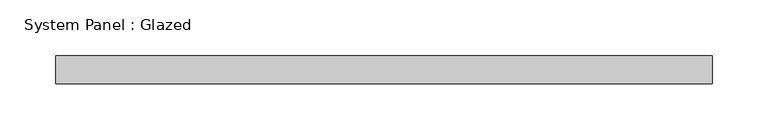
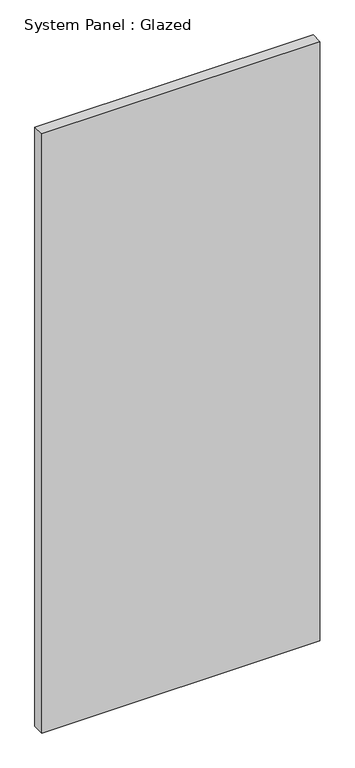
"""IFC4 building model written with IfcOpenShell, lengths in millimetres: plate geometry, System Panel : Glazed."""

from ifc_helpers import new_model, si_unit, origin, origin_with_axes, place, context, project, spatial, polyline, outline, extrude, source, transform, mapped, element, save


def system_panel_glazed_a22ed96f(model_context):
    return source(origin(), model_context, "Body", "SweptSolid", [
        extrude(outline(polyline([(295.275, 19.05), (-295.275, 19.05), (-295.275, 44.45), (295.275, 44.45), (295.275, 19.05)])), origin_with_axes(), (0.0, 0.0, 1.0), 1345.0504916),
    ])


if __name__ == "__main__":
    model = new_model("IFC4")
    model_context = context("Model", 3, world=origin())
    ifc_project = project(units=[si_unit("LENGTHUNIT", "METRE", prefix="MILLI")], contexts=[model_context])
    site = spatial("IfcSite", under=ifc_project)
    building = spatial("IfcBuilding", under=site)
    placement = place(None, origin())
    system_panel_glazed_shape = system_panel_glazed_a22ed96f(model_context)
    element("IfcPlate", 1, ObjectType="System Panel : Glazed", at=placement, inside=building, context=model_context, shape_type="MappedRepresentation", body=[
        mapped(system_panel_glazed_shape, transform((0.0, 0.0, 0.0), x_axis=(1.0, 0.0, 0.0), y_axis=(0.0, 1.0, 0.0), z_axis=(0.0, 0.0, 1.0))),
    ])
    save(model, "model.ifc")

# Revit data of these elements
# Type "System Panel : Glazed"
#   Construction Type Id = "GSP4R"
#   Analytic Construction = "1/8 in Pilkington single glazing"
#   Visual Light Transmittance = 0.9
#   Solar Heat Gain Coefficient = 0.86
#   Heat Transfer Coefficient (U) = 1.18115 BTU/(h·ft²·°F)
#   Define Thermal Properties by = 1
# Element 1 (IfcPlate, "System Panel : Glazed")
#   Materials on its faces: "Glass"
# Materials
#   "Glass": class "Glass", colour RGB 0 128 192, transparency 0.75, Description = "Soda Lime Glass", Cost = 0
